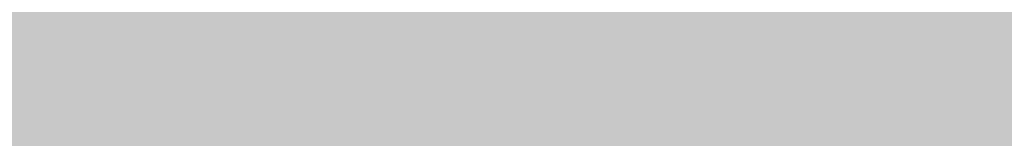
# Model space of a CAD drawing. Units: inches. Extents: x 2083 to 3317, y 1141 to 2115.
# Tile 129 of 256: x 3119.674 to 3123.979, y 1263.613 to 1264.131. Entities that reach past the tile are written whole.
import ezdxf

# ---------------------------------------------------------------- set-up
doc = ezdxf.new("R2010")
doc.units = ezdxf.units.IN
doc.layers.add('A-ANNO-DIMS', color=2, linetype='Continuous', lineweight=18)
doc.layers.add('A-WALL-PATT', color=251, linetype='Continuous', lineweight=13, true_color=0x636466)
doc.styles.get("Standard").update_dxf_attribs({"font": 'arial.ttf'})
doc.dimstyles.new('ISO-25', dxfattribs={"dimtxt": 12, "dimasz": 12, "dimexe": 1.25, "dimexo": 0.625, "dimtad": 1, "dimlunit": 3, "dimtxsty": 'Standard', "dimcen": 2.5, "dimadec": 0, "dimazin": 0, "dimtfac": 1, "dimtmove": 0, "dimatfit": 3, "dimfxl": 1, "dimarcsym": 0})

# ---------------------------------------------------------------- blocks, each defined once
blk = doc.blocks.new('*D26')
at = {"layer": 'A-ANNO-DIMS', "color": 0, "lineweight": -2, "transparency": 16777216}
for p, q in [((3088.9858, 1274.9151), (3088.9858, 1270.952)), ((3111.24, 1274.9151), (3111.24, 1270.952)), ((3076.9858, 1272.202), (2840.2624, 1272.202)), ((3111.24, 1272.202), (3088.9858, 1272.202)), ((3123.24, 1272.202), (3135.24, 1272.202))]:
    blk.add_line(p, q, dxfattribs=at)
at = {"layer": 'A-ANNO-DIMS', "color": 0, "transparency": 16777216}
for points in [[(3076.9858, 1274.202), (3076.9858, 1270.202), (3088.9858, 1272.202)], [(3123.24, 1274.202), (3123.24, 1270.202), (3111.24, 1272.202)]]:
    blk.add_solid(points, dxfattribs=at)
at = {"layer": 'Defpoints', "color": 0, "transparency": 16777216}
for p in [(3088.9858, 1275.5401), (3111.24, 1275.5401), (3088.9858, 1272.202)]:
    blk.add_point(p, dxfattribs=at)
at = {"layer": 'A-ANNO-DIMS', "color": 0, "transparency": 16777216, "insert": (2952.6241, 1279.0316), "char_height": 12, "attachment_point": 5}
blk.add_mtext('NIGHTSTAND 1\'-10 1/2" TYP.', dxfattribs=at)
blk = doc.blocks.new('*D27')
at = {"layer": 'A-ANNO-DIMS', "color": 0, "lineweight": -2, "transparency": 16777216}
for p, q in [((3114.5782, 1309.7943), (3114.5782, 1321.7943)), ((3111.865, 1297.7943), (3115.8282, 1297.7943)), ((3114.5782, 1297.7943), (3114.5782, 1275.5401)), ((3111.865, 1275.5401), (3115.8282, 1275.5401)), ((3114.5782, 1263.5401), (3114.5782, 1140.9886))]:
    blk.add_line(p, q, dxfattribs=at)
at = {"layer": 'A-ANNO-DIMS', "color": 0, "transparency": 16777216}
for points in [[(3112.5782, 1309.7943), (3116.5782, 1309.7943), (3114.5782, 1297.7943)], [(3112.5782, 1263.5401), (3116.5782, 1263.5401), (3114.5782, 1275.5401)]]:
    blk.add_solid(points, dxfattribs=at)
at = {"layer": 'Defpoints', "color": 0, "transparency": 16777216}
for p in [(3111.24, 1297.7943), (3111.24, 1275.5401), (3114.5782, 1275.5401)]:
    blk.add_point(p, dxfattribs=at)
at = {"layer": 'A-ANNO-DIMS', "color": 0, "transparency": 16777216, "insert": (3107.7485, 1196.2643), "char_height": 12, "attachment_point": 5, "rotation": 90}
blk.add_mtext('1\'-10 1/2" TYP.', dxfattribs=at)

msp = doc.modelspace()

# ---------------------------------------------------------------- hatches: boundary and pattern name
at = {"layer": 'A-WALL-PATT'}
h = msp.add_hatch(color=256, dxfattribs=at)
h.dxf.hatch_style = 1
h.paths.add_polyline_path([(3126.9598, 2020.7614), (2748.9598, 2020.7614), (2604.9598, 2020.7614), (2226.9598, 2020.7614), (2226.9598, 1702.7614), (2466.9598, 1702.7614), (2466.9598, 1582.7614), (2418.9598, 1582.7614), (2418.9598, 1477.7614), (2226.9598, 1477.7614), (2226.9598, 1263.2614), (2544.9598, 1263.2614), (2544.9598, 1411.7614), (2604.9598, 1411.7614), (2685.9598, 1411.7614), (2685.9598, 1420.7614), (2604.9598, 1420.7614), (2604.9598, 1573.7614), (2604.9598, 1702.7614), (2604.9598, 2011.7614), (2748.9598, 2011.7614), (2748.9598, 1702.7614), (2862.9598, 1702.7614), (2862.9598, 1621.7614), (2871.9598, 1621.7614), (2871.9598, 1702.7614), (2883.9598, 1702.7614), (2883.9598, 1706.9395, -0.026459), (2883.9598, 1711.7614), (2757.9598, 1711.7614), (2757.9598, 1807.7614), (2787.9598, 1807.7614), (2787.9598, 1812.2614), (2757.9598, 1812.2614), (2757.9598, 2011.7614), (2877.9598, 2011.7614), (2877.9598, 1812.2614), (2847.9598, 1812.2614), (2847.9598, 1807.7614), (2889.8357, 1807.7614), (2889.8357, 1812.2614), (2882.4598, 1812.2614), (2882.4598, 2011.7614), (3117.9598, 2011.7614), (3117.9598, 1812.2614), (2937.8357, 1812.2614), (2937.8357, 1807.7614), (2995.7098, 1807.7614), (2995.7098, 1796.1177), (3000.2098, 1796.1177), (3000.2098, 1807.7614), (3117.9598, 1807.7614), (3117.9598, 1711.7614), (3000.2098, 1711.7614), (3000.2098, 1760.1177), (2998.5727, 1760.1177, -0.020711), (2995.7098, 1760.1177), (2995.7098, 1711.7614), (2931.9598, 1711.7614), (2931.9598, 1702.7614), (3126.9598, 1702.7614)])
h.paths.add_polyline_path([(2471.4598, 2011.7614), (2471.4598, 1810.0114), (2462.7169, 1810.0114), (2462.7169, 1805.5114), (2505.9598, 1805.5114), (2505.9598, 1810.0114), (2475.9598, 1810.0114), (2475.9598, 2011.7614), (2595.9598, 2011.7614), (2595.9598, 1810.0114), (2565.9598, 1810.0114), (2565.9598, 1805.5114), (2595.9598, 1805.5114), (2595.9598, 1711.7614), (2235.9598, 1711.7614), (2235.9598, 1805.5114), (2353.7098, 1805.5114), (2353.7098, 1796.0542), (2358.2098, 1796.0542), (2358.2098, 1805.5114), (2414.7169, 1805.5114), (2414.7169, 1810.0114), (2235.9598, 1810.0114), (2235.9598, 2011.7614)], flags=16)
h.paths.add_polyline_path([(2270.2047, 1994.61), (2270.2047, 1970.61), (2246.2047, 1970.61), (2246.2047, 1994.61)], flags=0)
edge = h.paths.add_edge_path(flags=0)
edge.add_ellipse((2332.0274, 1899.7982), major_axis=(-3.043, 3.043), ratio=0.168252, start_angle=-161.3322, end_angle=-156.3071, ccw=False)
edge.add_ellipse((2333.082, 1898.7435), major_axis=(-1.0546, 1.0546), ratio=0.453532, start_angle=-123.371, end_angle=-94.1591)
edge = h.paths.add_edge_path(flags=0)
edge.add_ellipse((2332.0274, 1968.8763), major_axis=(3.043, 3.043), ratio=0.168252, start_angle=18.6678, end_angle=23.6929)
edge.add_spline(control_points=[(2332.9256, 1970.6911), (2332.2268, 1970.3361), (2330.8937, 1969.6589), (2328.4131, 1970.9321), (2327.2039, 1967.7487), (2324.7096, 1969.9556), (2322.5328, 1967.0124), (2320.0128, 1971.2958), (2317.6803, 1968.1578), (2316.0405, 1967.102), (2315.4269, 1966.8096)], knot_values=[0, 0, 0, 0, 2.267059, 4.324559, 6.685584, 8.878641, 11.121502, 14.300359, 17.755284, 19.732645, 19.732645, 19.732645, 19.732645], degree=3, periodic=0)
edge.add_ellipse((2332.0274, 1968.8763), major_axis=(3.043, 3.043), ratio=0.168252, start_angle=18.6678, end_angle=23.6929, ccw=False)
edge.add_ellipse((2333.082, 1969.9309), major_axis=(1.0546, 1.0546), ratio=0.453532, start_angle=56.629, end_angle=85.8409, ccw=False)
edge = h.paths.add_edge_path(flags=0)
edge.add_spline(control_points=[(2296.4283, 1967.9879), (2293.6278, 1965.3363), (2287.7036, 1959.7271), (2299.7439, 1949.9957), (2294.5326, 1935.6685), (2290.5732, 1920.6035), (2293.3941, 1909.9737), (2296.1854, 1904.9665)], knot_values=[0.099185, 0.099185, 0.099185, 0.099185, 0.345301, 0.619822, 0.982653, 1.386093, 1.810555, 1.810555, 1.810555, 1.810555], degree=3, periodic=0)
edge.add_spline(control_points=[(2296.1854, 1904.9665), (2297.3836, 1902.6193), (2298.001, 1901.9493), (2298.553, 1901.4682)], knot_values=[0.006246, 0.006246, 0.006246, 0.006246, 0.055476, 0.055476, 0.055476, 0.055476], degree=3, periodic=0)
edge.add_spline(control_points=[(2298.553, 1901.4682), (2297.2586, 1900.9232), (2295.2253, 1900.2321), (2293.0602, 1900.6142), (2292.1014, 1900.7884), (2292.0896, 1900.7906)], knot_values=[0.312835, 0.312835, 0.312835, 0.312835, 0.40178, 0.474987, 0.475903, 0.475903, 0.475903, 0.475903], degree=3, periodic=0)
edge.add_arc((2292.7936, 1904.6641), 3.937, 215.4209, 259.6982, ccw=False)
edge.add_spline(control_points=[(2289.5853, 1902.3823), (2289.4767, 1902.5351), (2289.3685, 1902.688), (2289.2609, 1902.8412)], knot_values=[0.102872, 0.102872, 0.102872, 0.102872, 0.116896, 0.116896, 0.116896, 0.116896], degree=3, periodic=0)
edge.add_spline(control_points=[(2289.2609, 1902.8412), (2288.6866, 1902.5502), (2287.64, 1902.0199), (2285.8813, 1901.874), (2283.853, 1901.5044), (2281.72, 1899.7105), (2278.467, 1899.4929), (2276.1571, 1901.8832), (2272.259, 1899.8041), (2267.7776, 1901.8432), (2262.2439, 1900.184), (2257.4149, 1901.7821), (2254.3184, 1900.7261), (2253.1783, 1900.3373)], knot_values=[0, 0, 0, 0, 1.907977, 3.477176, 5.261074, 7.972851, 11.680248, 13.717921, 16.939592, 22.789562, 27.502503, 33.595215, 37.145618, 37.145618, 37.145618, 37.145618], degree=3, periodic=0)
edge.add_line((2253.1783, 1900.3373), (2250.2442, 1902.8412))
edge.add_line((2250.2442, 1902.8412), (2250.2442, 1965.8333))
edge.add_line((2250.2442, 1965.8333), (2253.1783, 1968.3371))
edge.add_spline(control_points=[(2253.1783, 1968.3371), (2254.3184, 1967.9483), (2257.4149, 1966.8924), (2262.2439, 1968.4904), (2267.7776, 1966.8313), (2271.5267, 1968.5372), (2273.8759, 1967.8283), (2274.2067, 1967.7276)], knot_values=[0, 0, 0, 0, 0.09018, 0.244935, 0.364644, 0.513233, 0.537855, 0.537855, 0.537855, 0.537855], degree=3, periodic=0)
edge.add_arc((2274.3529, 1963.7933), 3.937, 72.0511, 92.1279, ccw=False)
edge.add_arc((2281.2969, 1985.23), 18.5963, 252.05113, 288.56572)
edge.add_arc((2292.3167, 1956.0289), 12.6461, 71.02679, 113.77822, ccw=False)
edge = h.paths.add_edge_path(flags=0)
edge.add_spline(control_points=[(2274.8994, 1951.8562), (2275.0662, 1951.6166), (2275.2327, 1951.3766), (2275.398, 1951.1359)], knot_values=[1.409916, 1.409916, 1.409916, 1.409916, 1.43159, 1.43159, 1.43159, 1.43159], degree=3, periodic=0)
edge.add_spline(control_points=[(2275.398, 1951.1359), (2275.7921, 1950.5619), (2276.1792, 1949.9838), (2276.5455, 1949.3971)], knot_values=[1.358238, 1.358238, 1.358238, 1.358238, 1.409916, 1.409916, 1.409916, 1.409916], degree=3, periodic=0)
edge.add_line((2276.5455, 1949.3971), (2277.4373, 1947.8622))
edge.add_spline(control_points=[(2277.4373, 1947.8622), (2276.3038, 1945.6731), (2274.6397, 1942.4269), (2274.6316, 1938.0939), (2272.7991, 1930.8515), (2274.3564, 1943.897), (2275.9477, 1947.9234), (2276.5455, 1949.3971)], knot_values=[0.005632, 0.005632, 0.005632, 0.005632, 0.186014, 0.266002, 0.357087, 0.59639, 0.739732, 0.739732, 0.739732, 0.739732], degree=3, periodic=0)
edge.add_spline(control_points=[(2276.5455, 1949.3971), (2276.1792, 1949.9838), (2275.7921, 1950.5619), (2275.398, 1951.1359)], knot_values=[1.358238, 1.358238, 1.358238, 1.358238, 1.409916, 1.409916, 1.409916, 1.409916], degree=3, periodic=0)
edge.add_spline(control_points=[(2275.398, 1951.1359), (2274.9425, 1950.0805), (2274.2078, 1948.0253), (2273.9346, 1944.8515), (2272.4685, 1937.6275), (2273.4662, 1945.6965), (2274.7006, 1951.0595), (2274.8994, 1951.8562)], knot_values=[0.104364, 0.104364, 0.104364, 0.104364, 0.189636, 0.269624, 0.36071, 0.600013, 0.644622, 0.644622, 0.644622, 0.644622], degree=3, periodic=0)
h.paths.add_polyline_path([(2269.1675, 1963.1276, -0.357527), (2268.1706, 1960.9764, -0.092561), (2268.1706, 1939.4363, -0.357527), (2269.1675, 1937.2851, -0.357527), (2267.0163, 1938.282, -0.164785), (2254.6856, 1938.282, -0.357527), (2252.5344, 1937.2851, -0.357527), (2253.5313, 1939.4363, -0.092561), (2253.5313, 1960.9764, -0.357527), (2252.5344, 1963.1276, -0.357527), (2254.6856, 1962.1307, -0.164785), (2267.0163, 1962.1307, -0.357527)], flags=0)
h.paths.add_polyline_path([(2248.8741, 1967.8018), (2248.8741, 1957.0277), (2249.4578, 1957.0277), (2249.4578, 1911.6468), (2248.8741, 1911.6468), (2248.8741, 1900.8727), (2246.5119, 1900.8727, 0.197327), (2244.1497, 1902.4569), (2244.1497, 1966.2176, 0.197327), (2246.5119, 1967.8018)], flags=0)
h.paths.add_polyline_path([(2269.1675, 1931.3893, -0.357527), (2268.1706, 1929.2381, -0.092561), (2268.1706, 1907.6981, -0.357527), (2269.1675, 1905.5469, -0.357527), (2267.0163, 1906.5438, -0.164785), (2254.6856, 1906.5438, -0.357527), (2252.5344, 1905.5469, -0.357527), (2253.5313, 1907.6981, -0.092561), (2253.5313, 1929.2381, -0.357527), (2252.5344, 1931.3893, -0.357527), (2254.6856, 1930.3925, -0.164785), (2267.0163, 1930.3925, -0.357527)], flags=0)
edge = h.paths.add_edge_path(flags=0)
edge.add_spline(control_points=[(2276.1969, 1906.7237), (2276.1681, 1909.0289), (2276.114, 1913.3719), (2270.5984, 1924.925), (2273.9052, 1919.0128), (2275.9217, 1916.2621), (2275.4746, 1912.4021), (2277.2579, 1910.3806), (2276.696, 1908.225), (2276.6462, 1906.813), (2276.6178, 1906.0084)], knot_values=[0, 0, 0, 0, 8.61026, 16.221274, 18.843057, 23.804898, 27.440828, 29.356102, 31.203478, 33.650687, 33.650687, 33.650687, 33.650687], degree=3, periodic=0)
edge.add_spline(control_points=[(2276.6178, 1906.0084), (2276.6233, 1905.6241), (2276.4977, 1904.6287), (2275.4418, 1903.8547), (2274.9373, 1903.0804), (2274.8591, 1902.8412)], knot_values=[0.156488, 0.156488, 0.156488, 0.156488, 0.184398, 0.231376, 0.250598, 0.250598, 0.250598, 0.250598], degree=3, periodic=0)
edge.add_line((2274.8591, 1902.8412), (2276.506, 1902.8412))
edge.add_spline(control_points=[(2276.506, 1902.8412), (2276.7883, 1903.0849), (2277.6651, 1904.1252), (2278.2495, 1904.3407), (2277.6539, 1908.5274), (2278.1557, 1906.2278), (2278.1005, 1905.2859), (2278.8467, 1904.069), (2277.8568, 1903.4149), (2277.8742, 1902.991), (2277.9036, 1902.8412)], knot_values=[0.059574, 0.059574, 0.059574, 0.059574, 0.080753, 0.103741, 0.16972, 0.176036, 0.207137, 0.240474, 0.262341, 0.27366, 0.27366, 0.27366, 0.27366], degree=3, periodic=0)
edge.add_line((2277.9036, 1902.8412), (2280.0298, 1902.8412))
edge.add_spline(control_points=[(2280.0298, 1902.8412), (2279.8882, 1903.0884), (2279.4993, 1903.9816), (2280.1523, 1905.9393), (2278.1036, 1909.6578), (2279.7624, 1907.1853), (2280.3279, 1904.8749), (2280.4851, 1903.4896), (2281.4633, 1903.2494), (2281.7583, 1902.9365), (2281.834, 1902.8412)], knot_values=[0.013856, 0.013856, 0.013856, 0.013856, 0.034874, 0.088867, 0.107879, 0.126738, 0.158714, 0.193757, 0.217487, 0.226722, 0.226722, 0.226722, 0.226722], degree=3, periodic=0)
edge.add_spline(control_points=[(2281.834, 1902.8412), (2281.7875, 1902.8267), (2281.647, 1902.783), (2281.3955, 1902.8595), (2281.0881, 1902.9852), (2280.7207, 1903.0609), (2280.3335, 1903.0257), (2280.1248, 1902.8989), (2280.0298, 1902.8412)], knot_values=[0, 0, 0, 0, 0.14413, 0.435517, 0.749276, 1.153046, 1.548371, 1.878348, 1.878348, 1.878348, 1.878348], degree=3, periodic=0)
edge.add_line((2280.0298, 1902.8412), (2277.9036, 1902.8412))
edge.add_spline(control_points=[(2277.9036, 1902.8412), (2277.8929, 1902.7959), (2277.8654, 1902.6796), (2277.6075, 1902.6875), (2277.2741, 1902.8007), (2276.8379, 1902.6198), (2276.5838, 1902.7893), (2276.506, 1902.8412)], knot_values=[0, 0, 0, 0, 0.127189, 0.326199, 0.628009, 1.24357, 1.515331, 1.515331, 1.515331, 1.515331], degree=3, periodic=0)
edge.add_line((2276.506, 1902.8412), (2274.8591, 1902.8412))
edge.add_spline(control_points=[(2274.8591, 1902.8412), (2274.8144, 1902.8986), (2274.7251, 1903.0134), (2274.4935, 1903.119), (2274.2443, 1902.9605), (2273.9371, 1903.1849), (2273.614, 1902.9831), (2273.4083, 1902.883), (2273.3223, 1902.8412)], knot_values=[0, 0, 0, 0, 0.21843, 0.436957, 0.687977, 0.990379, 1.398396, 1.69185, 1.69185, 1.69185, 1.69185], degree=3, periodic=0)
edge.add_spline(control_points=[(2273.3223, 1902.8412), (2273.6167, 1903.4457), (2274.274, 1904.5383), (2276.0272, 1904.5737), (2276.207, 1906.5836), (2276.1969, 1906.7237)], knot_values=[0.012227, 0.012227, 0.012227, 0.012227, 0.059472, 0.106218, 0.134458, 0.134458, 0.134458, 0.134458], degree=3, periodic=0)
h.paths.add_polyline_path([(2270.7761, 1897.7898), (2270.7761, 1873.7898), (2246.7761, 1873.7898), (2246.7761, 1897.7898)], flags=0)
h.paths.add_polyline_path([(2353.7098, 1760.0051), (2353.7098, 1760.0542), (2358.2098, 1760.0542, -0.033729)], flags=0)
h.paths.add_polyline_path([(2321.8191, 1737.5292), (2341.9953, 1737.5292, -0.414214), (2343.2033, 1736.3212), (2343.2033, 1721.0206, -0.414214), (2341.9953, 1719.8127), (2321.8191, 1719.8127, -0.414214), (2320.6112, 1721.0206), (2320.6112, 1736.3212, -0.414214)], flags=0)
h.paths.add_polyline_path([(2324.235, 1736.3212), (2339.5794, 1736.3212, -0.414214), (2341.9953, 1733.9053), (2341.9953, 1725.4497, -0.414214), (2339.5794, 1723.0338), (2333.6806, 1723.0338), (2333.8453, 1722.0455, -0.870646), (2335.4254, 1721.8259, -0.767327), (2333.9227, 1721.4232), (2331.291, 1721.4232, -0.767327), (2329.7883, 1721.8259, -0.870646), (2331.3684, 1722.0455), (2331.5331, 1723.0338), (2324.235, 1723.0338, -0.414214), (2321.8191, 1725.4497), (2321.8191, 1733.9053, -0.414214)], flags=0)
h.paths.add_polyline_path([(2570.4838, 1928.6154), (2589.6838, 1928.6154), (2590.1688, 1928.6154), (2590.1688, 1904.9934), (2570.4838, 1904.9934)], flags=0)
h.paths.add_polyline_path([(2574.4473, 1927.2638, -1), (2572.8288, 1927.2638, -1)], flags=0)
h.paths.add_polyline_path([(2573.0899, 1926.9409), (2573.925, 1927.776), (2574.1477, 1927.5533), (2573.3126, 1926.7182)], flags=0)
h.paths.add_polyline_path([(2578.7791, 1919.7296, -1), (2571.5917, 1919.7296, -1)], flags=0)
h.paths.add_polyline_path([(2578.3854, 1919.7296, -1), (2571.9854, 1919.7296, -1)], flags=0)
h.paths.add_polyline_path([(2331.5958, 1729.4762, -1), (2333.618, 1729.4762, -1)], flags=0)
h.paths.add_polyline_path([(2578.0342, 1927.2638, -1), (2576.4157, 1927.2638, -1)], flags=0)
h.paths.add_polyline_path([(2576.6889, 1927.5311), (2576.9116, 1927.7538), (2577.7467, 1926.9186), (2577.524, 1926.6959)], flags=0)
h.paths.add_polyline_path([(2578.1391, 1909.8595, -1), (2572.2317, 1909.8595, -1)], flags=0)
h.paths.add_polyline_path([(2577.7454, 1909.8595, -1), (2572.6254, 1909.8595, -1)], flags=0)
h.paths.add_polyline_path([(2583.7977, 1927.2638, -1), (2582.1792, 1927.2638, -1)], flags=0)
h.paths.add_polyline_path([(2582.7186, 1927.7538), (2583.5538, 1926.9186), (2583.3311, 1926.6959), (2582.4959, 1927.5311)], flags=0)
h.paths.add_polyline_path([(2582.4959, 1927.5311), (2582.7186, 1927.7538), (2583.5538, 1926.9186), (2583.3311, 1926.6959)], flags=0)
h.paths.add_polyline_path([(2587.7391, 1920.5296, -1), (2581.8317, 1920.5296, -1)], flags=0)
h.paths.add_polyline_path([(2587.3454, 1920.5296, -1), (2582.2254, 1920.5296, -1)], flags=0)
h.paths.add_polyline_path([(2587.3846, 1927.2638, -1), (2585.7661, 1927.2638, -1)], flags=0)
h.paths.add_polyline_path([(2586.082, 1926.9802), (2586.9172, 1927.8154), (2587.1399, 1927.5927), (2586.3047, 1926.7575)], flags=0)
h.paths.add_polyline_path([(2588.3791, 1910.6595, -1), (2581.1917, 1910.6595, -1)], flags=0)
h.paths.add_polyline_path([(2587.9854, 1910.6595, -1), (2581.5854, 1910.6595, -1)], flags=0)
h.paths.add_polyline_path([(2417.1677, 1729.4779), (2437.3439, 1729.4779, -0.414214), (2438.5519, 1728.2699), (2438.5519, 1712.9693, -0.414214), (2437.3439, 1711.7614), (2417.1677, 1711.7614, -0.414214), (2415.9598, 1712.9693), (2415.9598, 1728.2699, -0.414214)], flags=0)
h.paths.add_polyline_path([(2419.5836, 1728.2699), (2434.928, 1728.2699, -0.414214), (2437.3439, 1725.8541), (2437.3439, 1717.3984, -0.414214), (2434.928, 1714.9825), (2429.0292, 1714.9825), (2429.1939, 1713.9942, -0.870646), (2430.774, 1713.7746, -0.767327), (2429.2713, 1713.372), (2426.6396, 1713.372, -0.767327), (2425.1369, 1713.7746, -0.870646), (2426.717, 1713.9942), (2426.8817, 1714.9825), (2419.5836, 1714.9825, -0.414214), (2417.1677, 1717.3984), (2417.1677, 1725.8541, -0.414214)], flags=0)
h.paths.add_polyline_path([(2419.5836, 1728.2699), (2434.928, 1728.2699, -0.414214), (2437.3439, 1725.8541), (2437.3439, 1717.3984, -0.414214), (2434.928, 1714.9825), (2429.0292, 1714.9825), (2428.3581, 1719.009), (2427.5528, 1719.009), (2426.8817, 1714.9825), (2419.5836, 1714.9825, -0.414214), (2417.1677, 1717.3984), (2417.1677, 1725.8541, -0.414214)], flags=0)
h.paths.add_polyline_path([(2426.9444, 1721.4249, -1), (2428.9666, 1721.4249, -1)], flags=0)
h.paths.add_polyline_path([(2475.9598, 1702.7614), (2595.9598, 1702.7614), (2595.9598, 1582.7614), (2475.9598, 1582.7614)], flags=16)
h.paths.add_polyline_path([(2427.9598, 1573.7614), (2595.9598, 1573.7614), (2595.9598, 1468.7614), (2595.9598, 1420.7614), (2384.4598, 1420.7614), (2384.4598, 1468.7614), (2427.9598, 1468.7614)], flags=16)
h.paths.add_polyline_path([(2379.9598, 1468.7614), (2379.9598, 1420.7614), (2235.9598, 1420.7614), (2235.9598, 1468.7614)], flags=16)
h.paths.add_polyline_path([(2317.816, 1466.6958), (2337.9922, 1466.6958, -0.414214), (2339.2002, 1465.4878), (2339.2002, 1450.1872, -0.414214), (2337.9922, 1448.9792), (2317.816, 1448.9792, -0.414214), (2316.6081, 1450.1872), (2316.6081, 1465.4878, -0.414214)], flags=0)
h.paths.add_polyline_path([(2320.2319, 1465.4878), (2335.5763, 1465.4878, -0.414214), (2337.9922, 1463.0719), (2337.9922, 1454.6163, -0.414214), (2335.5763, 1452.2004), (2329.6775, 1452.2004), (2329.8422, 1451.212, -0.870646), (2331.4223, 1450.9925, -0.767327), (2329.9196, 1450.5898), (2327.2879, 1450.5898, -0.767327), (2325.7852, 1450.9925, -0.870646), (2327.3653, 1451.212), (2327.53, 1452.2004), (2320.2319, 1452.2004, -0.414214), (2317.816, 1454.6163), (2317.816, 1463.0719, -0.414214)], flags=0)
h.paths.add_polyline_path([(2320.2319, 1465.4878), (2335.5763, 1465.4878, -0.414214), (2337.9922, 1463.0719), (2337.9922, 1454.6163, -0.414214), (2335.5763, 1452.2004), (2329.6775, 1452.2004), (2329.0064, 1456.2269), (2328.2011, 1456.2269), (2327.53, 1452.2004), (2320.2319, 1452.2004, -0.414214), (2317.816, 1454.6163), (2317.816, 1463.0719, -0.414214)], flags=0)
h.paths.add_polyline_path([(2327.5926, 1458.6428, -1), (2329.6148, 1458.6428, -1)], flags=0)
h.paths.add_polyline_path([(2244.4117, 1433.3405), (2241.9209, 1433.3405, -0.414214), (2240.0179, 1435.2435), (2240.0179, 1440.9528, -0.414211), (2241.9209, 1442.8559), (2244.4117, 1442.8559, -1.976472)], flags=0)
h.paths.add_polyline_path([(2245.3569, 1434.3975, -0.414214), (2245.3569, 1441.7988, -2.144098)], flags=0)
h.paths.add_polyline_path([(2535.9598, 1416.2614), (2535.9598, 1272.2614), (2235.9598, 1272.2614), (2235.9598, 1416.2614)], flags=16)
h.paths.add_polyline_path([(2260.1196, 1384.2928), (2260.1196, 1362.0386), (2237.8654, 1362.0386), (2237.8654, 1384.2928)], flags=0)
edge = h.paths.add_edge_path(flags=0)
edge.add_line((2318.2518, 1362.0933), (2318.1458, 1362.001))
edge.add_ellipse((2317.4451, 1360.431), major_axis=(2.8216, 2.8216), ratio=0.168252, start_angle=18.6678, end_angle=20.9481, ccw=False)
edge.add_ellipse((2318.423, 1361.409), major_axis=(0.9779, 0.9779), ratio=0.453532, start_angle=56.629, end_angle=70.2262, ccw=False)
edge = h.paths.add_edge_path(flags=0)
edge.add_line((2319.1074, 1295.5711), (2319.015, 1295.6771))
edge.add_ellipse((2317.4451, 1296.3778), major_axis=(-2.8216, 2.8216), ratio=0.168252, start_angle=-161.3322, end_angle=-159.0519, ccw=False)
edge.add_ellipse((2318.423, 1295.3999), major_axis=(-0.9779, 0.9779), ratio=0.453532, start_angle=-123.371, end_angle=-109.7738)
edge = h.paths.add_edge_path(flags=0)
edge.add_spline(control_points=[(2284.2103, 1301.1702), (2284.5807, 1300.4447), (2284.8912, 1299.892), (2285.1596, 1299.461)], knot_values=[0.039066, 0.039066, 0.039066, 0.039066, 0.055476, 0.055476, 0.055476, 0.055476], degree=3, periodic=0)
edge.add_line((2285.1596, 1299.461), (2284.2103, 1301.1702))
edge = h.paths.add_edge_path(flags=0)
edge.add_line((2280.4125, 1297.298), (2283.37, 1297.0361))
edge.add_line((2283.37, 1297.0361), (2286.4057, 1297.9263))
edge.add_spline(control_points=[(2286.4057, 1297.9263), (2285.3055, 1297.4631), (2284.3448, 1297.1292), (2283.37, 1297.0361)], knot_values=[0.394369, 0.394369, 0.394369, 0.394369, 0.475903, 0.475903, 0.475903, 0.475903], degree=3, periodic=0)
edge.add_spline(control_points=[(2283.37, 1297.0361), (2283.2814, 1297.0277), (2282.3163, 1296.9573), (2281.3125, 1297.1345), (2280.4234, 1297.296), (2280.4125, 1297.298)], knot_values=[0.312835, 0.312835, 0.312835, 0.312835, 0.320246, 0.393453, 0.394369, 0.394369, 0.394369, 0.394369], degree=3, periodic=0)
edge = h.paths.add_edge_path(flags=0)
edge.add_line((2284.4356, 1359.6073), (2280.4463, 1355.328))
edge.add_line((2280.4463, 1355.328), (2279.58, 1351.0178))
edge.add_line((2279.58, 1351.0178), (2282.413, 1346.5804))
edge.add_spline(control_points=[(2282.413, 1346.5804), (2283.1533, 1345.5892), (2284.2529, 1344.0289), (2284.801, 1342.3872), (2284.9352, 1341.8055)], knot_values=[1.240098, 1.240098, 1.240098, 1.240098, 1.332892, 1.382712, 1.382712, 1.382712, 1.382712], degree=3, periodic=0)
edge.add_spline(control_points=[(2284.9352, 1341.8055), (2285.3191, 1340.1406), (2285.233, 1338.4092), (2284.9099, 1336.6541)], knot_values=[1.097484, 1.097484, 1.097484, 1.097484, 1.240098, 1.240098, 1.240098, 1.240098], degree=3, periodic=0)
edge.add_spline(control_points=[(2284.9099, 1336.6541), (2284.5868, 1334.899), (2284.0267, 1333.1203), (2283.4626, 1331.3606)], knot_values=[0.95487, 0.95487, 0.95487, 0.95487, 1.097484, 1.097484, 1.097484, 1.097484], degree=3, periodic=0)
edge.add_line((2283.4626, 1331.3606), (2281.8904, 1326.1534))
edge.add_line((2281.8904, 1326.1534), (2280.7563, 1321.0561))
edge.add_line((2280.7563, 1321.0561), (2280.2992, 1316.002))
edge.add_line((2280.2992, 1316.002), (2280.7159, 1310.9501))
edge.add_line((2280.7159, 1310.9501), (2282.0281, 1305.9721))
edge.add_line((2282.0281, 1305.9721), (2284.2103, 1301.1702))
edge.add_spline(control_points=[(2284.2103, 1301.1702), (2283.3407, 1302.7302), (2282.6119, 1304.3365), (2282.0281, 1305.9721)], knot_values=[0.099185, 0.099185, 0.099185, 0.099185, 0.241799, 0.241799, 0.241799, 0.241799], degree=3, periodic=0)
edge.add_spline(control_points=[(2282.0281, 1305.9721), (2281.4443, 1307.6078), (2281.0055, 1309.2728), (2280.7159, 1310.9501)], knot_values=[0.241799, 0.241799, 0.241799, 0.241799, 0.384413, 0.384413, 0.384413, 0.384413], degree=3, periodic=0)
edge.add_spline(control_points=[(2280.7159, 1310.9501), (2280.4332, 1312.5876), (2280.2894, 1314.277), (2280.2989, 1315.962), (2280.2992, 1316.002)], knot_values=[0.384413, 0.384413, 0.384413, 0.384413, 0.523647, 0.527028, 0.527028, 0.527028, 0.527028], degree=3, periodic=0)
edge.add_spline(control_points=[(2280.2992, 1316.002), (2280.3123, 1317.687), (2280.4779, 1319.3679), (2280.7563, 1321.0561)], knot_values=[0.527028, 0.527028, 0.527028, 0.527028, 0.669642, 0.669642, 0.669642, 0.669642], degree=3, periodic=0)
edge.add_spline(control_points=[(2280.7563, 1321.0561), (2281.0346, 1322.7443), (2281.4259, 1324.4396), (2281.8904, 1326.1534)], knot_values=[0.669642, 0.669642, 0.669642, 0.669642, 0.812256, 0.812256, 0.812256, 0.812256], degree=3, periodic=0)
edge.add_spline(control_points=[(2281.8904, 1326.1534), (2282.2644, 1327.5333), (2282.7879, 1329.2618), (2283.3528, 1331.0178), (2283.4626, 1331.3606)], knot_values=[0.812256, 0.812256, 0.812256, 0.812256, 0.927087, 0.95487, 0.95487, 0.95487, 0.95487], degree=3, periodic=0)
edge.add_line((2283.4626, 1331.3606), (2284.9099, 1336.6541))
edge.add_line((2284.9099, 1336.6541), (2284.9352, 1341.8055))
edge.add_line((2284.9352, 1341.8055), (2282.413, 1346.5804))
edge.add_spline(control_points=[(2282.413, 1346.5804), (2281.2751, 1348.1038), (2280.0784, 1349.5703), (2279.58, 1351.0178)], knot_values=[1.382712, 1.382712, 1.382712, 1.382712, 1.525326, 1.525326, 1.525326, 1.525326], degree=3, periodic=0)
edge.add_spline(control_points=[(2279.58, 1351.0178), (2279.4433, 1351.4147), (2279.1363, 1352.8569), (2279.7352, 1354.2904), (2280.4463, 1355.328)], knot_values=[1.525326, 1.525326, 1.525326, 1.525326, 1.564439, 1.667941, 1.667941, 1.667941, 1.667941], degree=3, periodic=0)
edge.add_spline(control_points=[(2280.4463, 1355.328), (2281.4261, 1356.7578), (2282.9308, 1358.1826), (2284.4356, 1359.6073)], knot_values=[1.667941, 1.667941, 1.667941, 1.667941, 1.810555, 1.810555, 1.810555, 1.810555], degree=3, periodic=0)
edge.add_arc((2280.6231, 1348.5182), 11.7262, 71.02679, 113.77822)
edge.add_arc((2270.4049, 1375.5952), 17.2436, 252.05113, 288.56572, ccw=False)
edge.add_arc((2263.966, 1355.7178), 3.6506, 72.0511, 92.1279)
edge.add_arc((2263.966, 1355.7178), 3.6506, 92.1279, 177.9851)
edge.add_spline(control_points=[(2260.3176, 1355.8462), (2260.2604, 1354.2207), (2260.5513, 1350.1865), (2262.9993, 1346.7663), (2264.4727, 1344.649)], knot_values=[1.43159, 1.43159, 1.43159, 1.43159, 1.564144, 1.770695, 1.770695, 1.770695, 1.770695], degree=3, periodic=0)
edge.add_line((2264.4727, 1344.649), (2264.9356, 1343.9825))
edge.add_spline(control_points=[(2263.801, 1340.2481), (2263.8432, 1340.5141), (2264.0672, 1341.7565), (2264.5127, 1343.0025), (2264.935, 1343.9811)], knot_values=[0.53657, 0.53657, 0.53657, 0.53657, 0.559349, 0.644622, 0.644622, 0.644622, 0.644622], degree=3, periodic=0)
edge.add_spline(control_points=[(2264.935, 1343.9811), (2265.1178, 1343.715), (2265.2989, 1343.4479), (2265.4768, 1343.1794)], knot_values=[1.384077, 1.384077, 1.384077, 1.384077, 1.409916, 1.409916, 1.409916, 1.409916], degree=3, periodic=0)
edge.add_spline(control_points=[(2265.4768, 1343.1794), (2265.6546, 1342.9108), (2265.8293, 1342.6408), (2265.9991, 1342.3688)], knot_values=[1.358238, 1.358238, 1.358238, 1.358238, 1.384077, 1.384077, 1.384077, 1.384077], degree=3, periodic=0)
edge.add_line((2265.9991, 1342.3688), (2266.826, 1340.9455))
edge.add_spline(control_points=[(2266.826, 1340.9455), (2268.8944, 1337.0897), (2271.3982, 1325.843), (2270.5162, 1310.5686), (2275.9194, 1301.8606), (2277.7895, 1299.1994)], knot_values=[0.116896, 0.116896, 0.116896, 0.116896, 0.472987, 1.050969, 1.313793, 1.313793, 1.313793, 1.313793], degree=3, periodic=0)
edge.add_spline(control_points=[(2277.7895, 1299.1994), (2277.8394, 1299.1285), (2277.8894, 1299.0575), (2277.9396, 1298.9866)], knot_values=[0.109884, 0.109884, 0.109884, 0.109884, 0.116896, 0.116896, 0.116896, 0.116896], degree=3, periodic=0)
edge.add_line((2277.9396, 1298.9866), (2277.7888, 1299.1991))
edge.add_spline(control_points=[(2277.7888, 1299.1991), (2277.2566, 1298.9294), (2276.2864, 1298.4379), (2275.0394, 1298.3344), (2274.3833, 1298.2389), (2274.2153, 1298.2093)], knot_values=[33.12187, 33.12187, 33.12187, 33.12187, 35.029056, 36.598255, 37.144827, 37.144827, 37.144827, 37.144827], degree=3, periodic=0)
edge.add_line((2274.2153, 1298.2093), (2273.0731, 1297.893))
edge.add_spline(control_points=[(2273.0731, 1297.893), (2272.3229, 1297.5798), (2271.0392, 1296.5105), (2269.2484, 1296.2261), (2268.4231, 1296.3747)], knot_values=[26.532584, 26.532584, 26.532584, 26.532584, 29.198919, 31.839101, 31.839101, 31.839101, 31.839101], degree=3, periodic=0)
edge.add_line((2268.4231, 1296.3747), (2263.8785, 1297.4575))
edge.add_spline(control_points=[(2263.8785, 1297.4575), (2263.5561, 1297.3594), (2261.8603, 1296.8387), (2260.2388, 1297.2824), (2258.9335, 1297.5165)], knot_values=[15.919551, 15.919551, 15.919551, 15.919551, 16.939592, 21.226067, 21.226067, 21.226067, 21.226067], degree=3, periodic=0)
edge.add_line((2258.9335, 1297.5165), (2254.0552, 1297.329))
edge.add_spline(control_points=[(2254.0552, 1297.329), (2253.7555, 1297.2958), (2252.1137, 1297.1652), (2250.4619, 1297.5442), (2249.1297, 1297.6679)], knot_values=[5.306517, 5.306517, 5.306517, 5.306517, 6.276435, 10.613034, 10.613034, 10.613034, 10.613034], degree=3, periodic=0)
edge.add_line((2249.1297, 1297.6679), (2244.3316, 1296.8778))
edge.add_line((2244.3316, 1296.8778), (2241.611, 1299.1994))
edge.add_line((2241.611, 1299.1994), (2241.611, 1357.6094))
edge.add_line((2241.611, 1357.6094), (2244.3316, 1359.9311))
edge.add_line((2244.3316, 1359.9311), (2252.7288, 1359.5427))
edge.add_spline(control_points=[(2252.7288, 1359.5427), (2252.8709, 1359.5464), (2253.3057, 1359.5482), (2253.7398, 1359.5143), (2254.0317, 1359.4824)], knot_values=[0.233291, 0.233291, 0.233291, 0.233291, 0.244935, 0.268927, 0.268927, 0.268927, 0.268927], degree=3, periodic=0)
edge.add_line((2254.0317, 1359.4824), (2259.5872, 1359.4164))
edge.add_spline(control_points=[(2259.5872, 1359.4164), (2260.6771, 1359.6285), (2262.0732, 1359.897), (2263.5237, 1359.4593), (2263.8304, 1359.366)], knot_values=[0.422516, 0.422516, 0.422516, 0.422516, 0.513233, 0.537855, 0.537855, 0.537855, 0.537855], degree=3, periodic=0)
edge.add_arc((2263.966, 1355.7178), 3.6506, 72.0511, 92.1279, ccw=False)
edge.add_arc((2270.4049, 1375.5952), 17.2436, 252.05113, 288.56572)
edge.add_arc((2280.6231, 1348.5182), 11.7262, 71.02679, 113.77822, ccw=False)
h.paths.add_polyline_path([(2240.3405, 1359.4347), (2240.3405, 1349.4444), (2240.8818, 1349.4444), (2240.8818, 1307.3645), (2240.3405, 1307.3645), (2240.3405, 1297.3741), (2238.1502, 1297.3741, 0.197327), (2235.9598, 1298.8431), (2235.9598, 1357.9657, 0.197327), (2238.1502, 1359.4347)], flags=0)
h.paths.add_polyline_path([(2259.1578, 1355.1005, -0.357527), (2258.2334, 1353.1058, -0.092561), (2258.2334, 1333.1326, -0.357527), (2259.1578, 1331.1379, -0.357527), (2257.1631, 1332.0622, -0.164785), (2245.7293, 1332.0622, -0.357527), (2243.7346, 1331.1379, -0.357527), (2244.6589, 1333.1326, -0.092561), (2244.6589, 1353.1058, -0.357527), (2243.7346, 1355.1005, -0.357527), (2245.7293, 1354.1761, -0.164785), (2257.1631, 1354.1761, -0.357527)], flags=0)
edge = h.paths.add_edge_path(flags=0)
edge.add_line((2265.9991, 1342.3688), (2266.826, 1340.9455))
edge.add_line((2266.826, 1340.9455), (2265.3076, 1337.8141))
edge.add_line((2265.3076, 1337.8141), (2264.3582, 1334.6529))
edge.add_line((2264.3582, 1334.6529), (2264.262, 1333.7997))
edge.add_spline(control_points=[(2264.262, 1333.7997), (2264.2084, 1333.1871), (2264.1621, 1332.3655), (2264.0071, 1331.4139), (2263.969, 1331.2018)], knot_values=[0.464444, 0.464444, 0.464444, 0.464444, 0.516691, 0.531608, 0.531608, 0.531608, 0.531608], degree=3, periodic=0)
edge.add_spline(control_points=[(2263.969, 1331.2018), (2263.7745, 1330.1189), (2263.4244, 1328.7908), (2263.2574, 1328.5307), (2263.234, 1328.5146)], knot_values=[0.372682, 0.372682, 0.372682, 0.372682, 0.44885, 0.464444, 0.464444, 0.464444, 0.464444], degree=3, periodic=0)
edge.add_spline(control_points=[(2263.234, 1328.5146), (2263.0964, 1328.4202), (2263.1312, 1329.3015), (2263.275, 1330.6157)], knot_values=[0.280919, 0.280919, 0.280919, 0.280919, 0.372682, 0.372682, 0.372682, 0.372682], degree=3, periodic=0)
edge.add_spline(control_points=[(2263.275, 1330.6157), (2263.4187, 1331.93), (2263.6715, 1333.6773), (2263.9699, 1335.315)], knot_values=[0.189157, 0.189157, 0.189157, 0.189157, 0.280919, 0.280919, 0.280919, 0.280919], degree=3, periodic=0)
edge.add_spline(control_points=[(2263.9699, 1335.315), (2264.1005, 1336.0322), (2264.4188, 1337.6219), (2264.7548, 1338.8644), (2264.9474, 1339.4911)], knot_values=[0.097394, 0.097394, 0.097394, 0.097394, 0.137578, 0.189157, 0.189157, 0.189157, 0.189157], degree=3, periodic=0)
edge.add_spline(control_points=[(2264.9474, 1339.4911), (2265.29, 1340.6061), (2265.6442, 1341.494), (2265.9991, 1342.3688)], knot_values=[0.005632, 0.005632, 0.005632, 0.005632, 0.097394, 0.097394, 0.097394, 0.097394], degree=3, periodic=0)
h.paths.add_polyline_path([(2259.1578, 1325.671, -0.357527), (2258.2334, 1323.6763, -0.092561), (2258.2334, 1303.7031, -0.357527), (2259.1578, 1301.7084, -0.357527), (2257.1631, 1302.6327, -0.164785), (2245.7293, 1302.6327, -0.357527), (2243.7346, 1301.7084, -0.357527), (2244.6589, 1303.7031, -0.092561), (2244.6589, 1323.6763, -0.357527), (2243.7346, 1325.671, -0.357527), (2245.7293, 1324.7466, -0.164785), (2257.1631, 1324.7466, -0.357527)], flags=0)
edge = h.paths.add_edge_path(flags=0)
edge.add_spline(control_points=[(2261.7089, 1317.3114), (2261.6795, 1317.4176), (2261.7619, 1317.3885), (2262.4907, 1316.0899), (2262.9622, 1315.3009)], knot_values=[14.955861, 14.955861, 14.955861, 14.955861, 16.221274, 18.694826, 18.694826, 18.694826, 18.694826], degree=3, periodic=0)
edge.add_spline(control_points=[(2262.9622, 1315.3009), (2262.9904, 1315.2536), (2263.7021, 1314.0674), (2264.349, 1313.1272), (2264.7301, 1312.1642)], knot_values=[18.694826, 18.694826, 18.694826, 18.694826, 18.843057, 22.433791, 22.433791, 22.433791, 22.433791], degree=3, periodic=0)
edge.add_spline(control_points=[(2264.7301, 1312.1642), (2264.8756, 1311.7964), (2265.1769, 1310.7698), (2265.1431, 1309.5593), (2265.2477, 1308.8242)], knot_values=[22.433791, 22.433791, 22.433791, 22.433791, 23.804898, 26.172756, 26.172756, 26.172756, 26.172756], degree=3, periodic=0)
edge.add_line((2265.2477, 1308.8242), (2265.8508, 1307.1719))
edge.add_spline(control_points=[(2265.8508, 1307.1719), (2266.065, 1306.8217), (2266.3844, 1306.3322), (2266.4244, 1305.7805), (2266.4204, 1305.6112)], knot_values=[28.062562, 28.062562, 28.062562, 28.062562, 29.356102, 29.911721, 29.911721, 29.911721, 29.911721], degree=3, periodic=0)
edge.add_spline(control_points=[(2266.4204, 1305.6112), (2266.4161, 1305.4326), (2266.394, 1305.25), (2266.3648, 1305.0659)], knot_values=[29.911721, 29.911721, 29.911721, 29.911721, 30.497837, 30.497837, 30.497837, 30.497837], degree=3, periodic=0)
edge.add_line((2266.3648, 1305.0659), (2266.0662, 1302.1363))
edge.add_spline(control_points=[(2266.0662, 1302.1363), (2266.0712, 1301.78), (2265.9981, 1301.2), (2265.6633, 1300.759), (2265.5089, 1300.5859)], knot_values=[0.156488, 0.156488, 0.156488, 0.156488, 0.184398, 0.203543, 0.203543, 0.203543, 0.203543], degree=3, periodic=0)
edge.add_line((2265.5089, 1300.5859), (2264.4353, 1299.1994))
edge.add_line((2264.4353, 1299.1994), (2265.9624, 1299.1994))
edge.add_line((2265.9624, 1299.1994), (2267.336, 1301.1753))
edge.add_line((2267.336, 1301.1753), (2267.3117, 1301.9862))
edge.add_spline(control_points=[(2267.3117, 1301.9862), (2267.2611, 1302.8624), (2267.1602, 1303.7371), (2267.2715, 1303.3259)], knot_values=[0.126229, 0.126229, 0.126229, 0.126229, 0.166617, 0.166617, 0.166617, 0.166617], degree=3, periodic=0)
edge.add_spline(control_points=[(2267.2715, 1303.3259), (2267.28, 1303.2943), (2267.3098, 1303.1754), (2267.3735, 1302.8836), (2267.4061, 1302.6828), (2267.4179, 1302.601)], knot_values=[0.166617, 0.166617, 0.166617, 0.166617, 0.16972, 0.176036, 0.180765, 0.180765, 0.180765, 0.180765], degree=3, periodic=0)
edge.add_spline(control_points=[(2267.7439, 1300.9875), (2267.6876, 1301.1509), (2267.4805, 1301.6567), (2267.4838, 1302.1448), (2267.4179, 1302.601)], knot_values=[0.180765, 0.180765, 0.180765, 0.180765, 0.193767, 0.220139, 0.220139, 0.220139, 0.220139], degree=3, periodic=0)
edge.add_line((2267.4179, 1302.601), (2267.7439, 1300.9875))
edge.add_spline(control_points=[(2267.7439, 1300.9875), (2267.832, 1300.7319), (2267.932, 1300.3099), (2267.5548, 1299.9745), (2267.4294, 1299.8292)], knot_values=[0.220139, 0.220139, 0.220139, 0.220139, 0.240474, 0.25489, 0.25489, 0.25489, 0.25489], degree=3, periodic=0)
edge.add_line((2267.4294, 1299.8292), (2267.2584, 1299.1994))
edge.add_line((2267.2584, 1299.1994), (2269.23, 1299.1994))
edge.add_spline(control_points=[(2269.23, 1299.1994), (2269.0987, 1299.4287), (2268.8428, 1300.0163), (2269.0116, 1300.9159), (2268.9468, 1301.6607)], knot_values=[0.013856, 0.013856, 0.013856, 0.013856, 0.034874, 0.067073, 0.067073, 0.067073, 0.067073], degree=3, periodic=0)
edge.add_line((2268.9468, 1301.6607), (2268.4316, 1303.6031))
edge.add_spline(control_points=[(2268.4316, 1303.6031), (2268.1756, 1304.1924), (2267.5962, 1305.2513), (2268.0407, 1304.6232), (2268.2514, 1304.2824)], knot_values=[0.090155, 0.090155, 0.090155, 0.090155, 0.107879, 0.120289, 0.120289, 0.120289, 0.120289], degree=3, periodic=0)
edge.add_spline(control_points=[(2268.2514, 1304.2824), (2268.3609, 1304.1053), (2269.0578, 1302.918), (2269.3827, 1301.5904), (2269.5214, 1300.7759), (2269.5752, 1300.5558)], knot_values=[0.120289, 0.120289, 0.120289, 0.120289, 0.126738, 0.158714, 0.173506, 0.173506, 0.173506, 0.173506], degree=3, periodic=0)
edge.add_line((2269.5752, 1300.5558), (2270.6858, 1299.4213))
edge.add_spline(control_points=[(2270.6858, 1299.4213), (2270.7672, 1299.3573), (2270.8379, 1299.2814), (2270.9029, 1299.1994)], knot_values=[0.21816, 0.21816, 0.21816, 0.21816, 0.226722, 0.226722, 0.226722, 0.226722], degree=3, periodic=0)
edge.add_line((2270.9372, 1299.1929), (2270.9029, 1299.1994))
edge.add_spline(control_points=[(2270.9029, 1299.1994), (2270.8598, 1299.186), (2270.7295, 1299.1455), (2270.4963, 1299.2164), (2270.2717, 1299.3083), (2270.121, 1299.348), (2270.0633, 1299.3596)], knot_values=[0.939174, 0.939174, 0.939174, 0.939174, 1.083304, 1.374691, 1.68845, 1.878348, 1.878348, 1.878348, 1.878348], degree=3, periodic=0)
edge.add_line((2270.0633, 1299.3596), (2269.23, 1299.1994))
edge.add_line((2269.23, 1299.1994), (2267.2584, 1299.1994))
edge.add_spline(control_points=[(2267.2584, 1299.1994), (2267.2484, 1299.1574), (2267.223, 1299.0497), (2266.9838, 1299.0569), (2266.8092, 1299.1162), (2266.6769, 1299.1091), (2266.6365, 1299.1048)], knot_values=[0.757665, 0.757665, 0.757665, 0.757665, 0.884854, 1.083864, 1.385675, 1.515331, 1.515331, 1.515331, 1.515331], degree=3, periodic=0)
edge.add_spline(control_points=[(2266.6365, 1299.1048), (2266.4852, 1299.0888), (2266.2358, 1299.0171), (2266.0346, 1299.1513), (2265.9624, 1299.1994)], knot_values=[0, 0, 0, 0, 0.485905, 0.757665, 0.757665, 0.757665, 0.757665], degree=3, periodic=0)
edge.add_line((2265.9624, 1299.1994), (2264.4353, 1299.1994))
edge.add_line((2264.4353, 1299.1994), (2263.8584, 1299.3671))
edge.add_spline(control_points=[(2263.8584, 1299.3671), (2263.8189, 1299.3709), (2263.7795, 1299.3857), (2263.7401, 1299.4015)], knot_values=[0.845925, 0.845925, 0.845925, 0.845925, 0.978627, 0.978627, 0.978627, 0.978627], degree=3, periodic=0)
edge.add_line((2263.7218, 1299.3964), (2263.0103, 1299.1994))
edge.add_spline(control_points=[(2263.0103, 1299.1994), (2263.2458, 1299.6829), (2263.506, 1300.1281), (2263.8735, 1300.408)], knot_values=[0.012227, 0.012227, 0.012227, 0.012227, 0.052971, 0.052971, 0.052971, 0.052971], degree=3, periodic=0)
edge.add_spline(control_points=[(2263.8735, 1300.408), (2263.9321, 1300.4527), (2264.0842, 1300.553), (2264.2552, 1300.6242), (2264.3597, 1300.6647)], knot_values=[0.052971, 0.052971, 0.052971, 0.052971, 0.059472, 0.069086, 0.069086, 0.069086, 0.069086], degree=3, periodic=0)
edge.add_line((2264.3597, 1300.6647), (2265.1419, 1301.0778))
edge.add_line((2265.1419, 1301.0778), (2265.6758, 1302.7996))
edge.add_line((2265.6758, 1302.7996), (2265.5407, 1305.7041))
edge.add_line((2265.5407, 1305.7041), (2264.8031, 1309.3277))
edge.add_line((2264.8031, 1309.3277), (2263.0405, 1314.0918))
edge.add_spline(control_points=[(2263.0405, 1314.0918), (2262.3836, 1315.6714), (2261.796, 1316.9977), (2261.7089, 1317.3114)], knot_values=[11.216896, 11.216896, 11.216896, 11.216896, 14.955861, 14.955861, 14.955861, 14.955861], degree=3, periodic=0)
h.paths.add_polyline_path([(2871.9598, 1416.2614), (2895.91, 1416.2614), (2895.91, 1420.7614), (2871.9598, 1420.7614), (2871.9598, 1501.7614), (2862.9598, 1501.7614), (2862.9598, 1420.7614), (2805.9598, 1420.7614), (2805.9598, 1411.7614), (2862.9598, 1411.7614), (2862.9598, 1263.2614), (3126.9598, 1263.2614), (3126.9598, 1411.7614), (3126.9598, 1486.7614), (2943.9598, 1486.7614), (2943.9598, 1477.7614), (2967.8603, 1477.7614), (2967.8603, 1420.7614), (2943.91, 1420.7614), (2943.91, 1416.2614), (3117.9598, 1416.2614), (3117.9598, 1420.7614), (2972.3603, 1420.7614), (2972.3603, 1477.7614), (3117.9598, 1477.7614), (3117.9598, 1420.7614), (3117.9598, 1272.2614), (2871.9598, 1272.2614)], flags=0)
h.paths.add_polyline_path([(2457.1256, 1485.9425), (2527.6027, 1485.9425), (2527.6027, 1537.6357), (2457.1256, 1537.6357)], flags=8)
h.paths.add_polyline_path([(2481.0051, 1609.9818), (2590.7658, 1609.9818), (2590.7658, 1682.0034), (2481.0051, 1682.0034)], flags=8)
h.paths.add_polyline_path([(2483.085, 1729.1268), (2553.562, 1729.1268), (2553.562, 1780.82), (2483.085, 1780.82)], flags=8)
h = msp.add_hatch(color=256, dxfattribs=at)
h.dxf.hatch_style = 1
h.paths.add_polyline_path([(3126.9598, 1486.7614), (2943.9598, 1486.7614), (2943.9598, 1477.7614), (2967.8603, 1477.7614), (2967.8603, 1420.7614), (2943.91, 1420.7614), (2943.91, 1416.2614), (3117.9598, 1416.2614), (3117.9598, 1420.7614), (2972.3603, 1420.7614), (2972.3603, 1477.7614), (3117.9598, 1477.7614), (3117.9598, 1420.7614), (3117.9598, 1272.2614), (2871.9598, 1272.2614), (2871.9598, 1416.2614), (2895.91, 1416.2614), (2895.91, 1420.7614), (2871.9598, 1420.7614), (2871.9598, 1501.7614), (2862.9598, 1501.7614), (2862.9598, 1420.7614), (2805.9598, 1420.7614), (2805.9598, 1411.7614), (2862.9598, 1411.7614), (2862.9598, 1263.2614), (3126.9598, 1263.2614), (3126.9598, 1411.7614)])

# ---------------------------------------------------------------- dimensions: what is measured, and where the dimension line sits
at = {"layer": 'A-ANNO-DIMS'}
for base, p1, p2, angle, text, picture, middle in [((3114.5782, 1275.5401), (3111.24, 1297.7943), (3111.24, 1275.5401), 270, '<> TYP.', '*D27', (3107.7485, 1196.2643)), ((3088.9858, 1272.202), (3111.24, 1275.5401), (3088.9858, 1275.5401), 180, 'NIGHTSTAND <> TYP.', '*D26', (2952.6241, 1279.0316))]:
    dim = msp.add_linear_dim(base=base, p1=p1, p2=p2, angle=angle, text=text, dimstyle='ISO-25', override={"dimdec": 1, "dimlfac": 1, "dimrnd": 0, "dimzin": 1, "dimdsep": 46, "dimlunit": 4, "dimfrac": 2}, dxfattribs=at)
    dim.commit()
    dim.dimension.update_dxf_attribs({"geometry": picture, "text_midpoint": middle})

doc.saveas('drawing.dxf')
